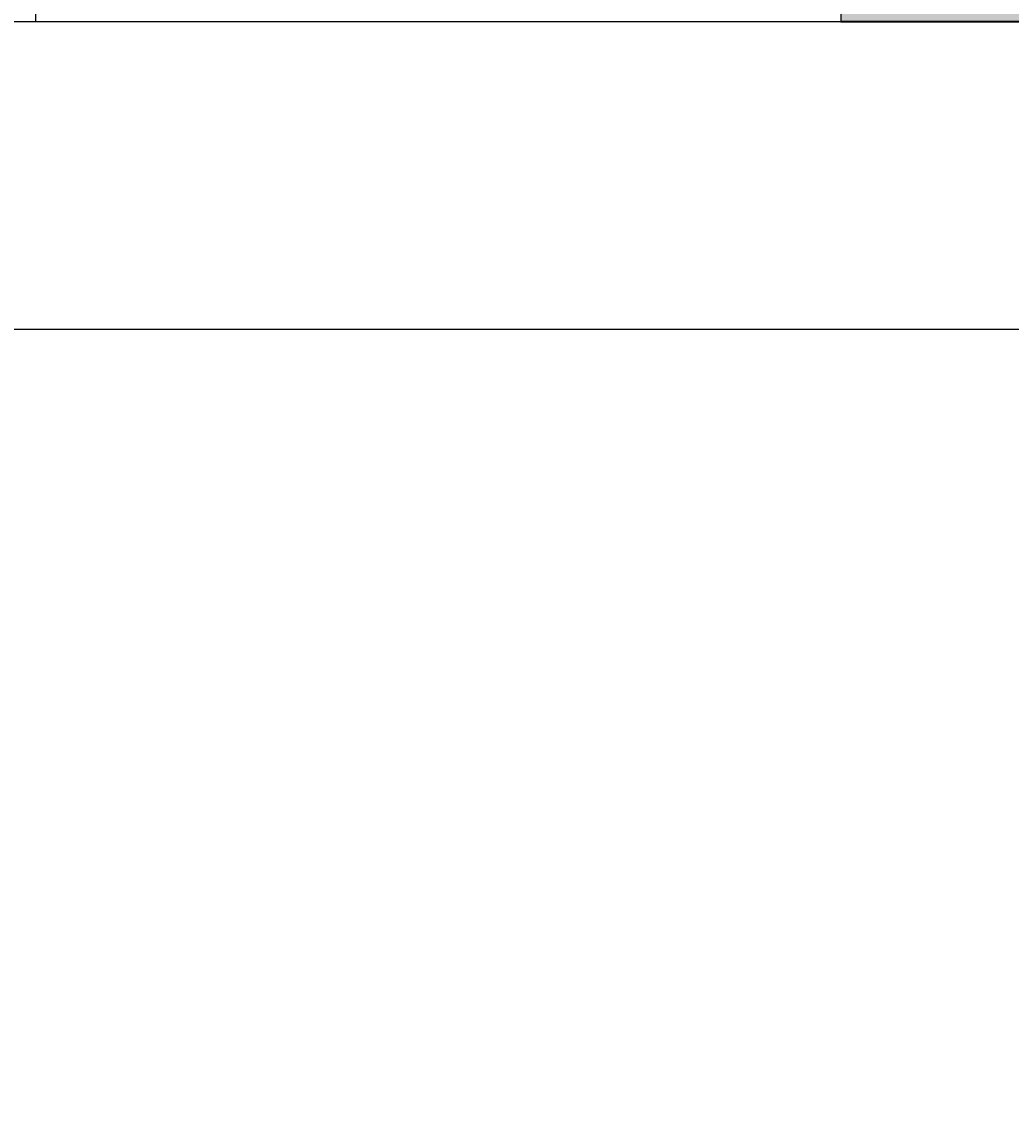
# Model space of a CAD drawing. Units: inches. Extents: x 1998 to 2588, y 1139 to 1977.
# Tile 98 of 134: x 2371 to 2397, y 1608 to 1637. Entities that reach past the tile are written whole.
import ezdxf

# ---------------------------------------------------------------- set-up
doc = ezdxf.new("R2010")
doc.units = ezdxf.units.IN
for name, color, linetype, lineweight in [('A-ANNO-DIMS', 2, 'Continuous', 18), ('A-WALL-PATT', 252, 'Continuous', 13), ('DOOR', 52, 'Continuous', 25), ('WALL', 200, 'Continuous', 35)]:
    doc.layers.add(name, color=color, linetype=linetype, lineweight=lineweight)
doc.styles.get("Standard").update_dxf_attribs({"font": 'arial.ttf'})
doc.dimstyles.get("Standard").update_dxf_attribs({"dimtxt": 0.18, "dimasz": 0.18, "dimexe": 0.18, "dimexo": 0.0625, "dimgap": 0.09, "dimtad": 0, "dimtih": 1, "dimtoh": 1, "dimdec": 4, "dimzin": 0, "dimdsep": 46, "dimtxsty": 'Standard', "dimcen": 0.09, "dimadec": 0, "dimazin": 0, "dimtfac": 1, "dimtdec": 4, "dimtofl": 0, "dimtmove": 0, "dimatfit": 3, "dimfxl": 1, "dimtolj": 1, "dimtzin": 0, "dimarcsym": 0})

# ---------------------------------------------------------------- blocks, each defined once
blk = doc.blocks.new('*U2')
for p, q in [((0, 0), (0, -6)), ((40, 0), (40, -6))]:
    blk.add_line(p, q)
blk.add_lwpolyline([(0, 0), (0, 40), (1.75, 40), (1.75, 0)], close=True)
blk.add_arc((0, 0), 40, 0, 90)
blk = doc.blocks.new('*D30')
at = {"layer": 'A-ANNO-DIMS', "color": 0, "lineweight": -2, "transparency": 16777216}
for p, q in [((2407.91, 1636.732), (1997.843, 1636.732)), ((1998.023, 1636.552), (1998.023, 1615.913)), ((1998.023, 1594.912), (1998.023, 1615.552)), ((2407.91, 1594.732), (1997.843, 1594.732))]:
    blk.add_line(p, q, dxfattribs=at)
at = {"layer": 'A-ANNO-DIMS', "color": 0, "transparency": 16777216}
for points in [[(1997.993, 1636.552), (1998.053, 1636.552), (1998.023, 1636.732)], [(1997.993, 1594.912), (1998.053, 1594.912), (1998.023, 1594.732)]]:
    blk.add_solid(points, dxfattribs=at)
at = {"layer": 'Defpoints', "color": 0, "transparency": 16777216}
for p in [(1998.023, 1636.732), (2407.973, 1636.732), (2407.973, 1594.732)]:
    blk.add_point(p, dxfattribs=at)
at = {"layer": 'A-ANNO-DIMS', "color": 0, "transparency": 16777216, "insert": (1998.023, 1615.732), "char_height": 0.18, "attachment_point": 5}
blk.add_mtext('\\A1;42', dxfattribs=at)
blk = doc.blocks.new('*D39')
at = {"layer": 'A-ANNO-DIMS', "color": 0, "lineweight": -2, "transparency": 16777216}
for p, q in [((2115.035, 1628.742), (2588.309, 1628.742)), ((2588.129, 1628.562), (2588.129, 1612.685)), ((2588.129, 1596.444), (2588.129, 1612.321)), ((2115.035, 1596.264), (2588.309, 1596.264))]:
    blk.add_line(p, q, dxfattribs=at)
at = {"layer": 'A-ANNO-DIMS', "color": 0, "transparency": 16777216}
for points in [[(2588.099, 1628.562), (2588.159, 1628.562), (2588.129, 1628.742)], [(2588.099, 1596.444), (2588.159, 1596.444), (2588.129, 1596.264)]]:
    blk.add_solid(points, dxfattribs=at)
at = {"layer": 'Defpoints', "color": 0, "transparency": 16777216}
for p in [(2114.973, 1628.742), (2588.129, 1628.742), (2114.973, 1596.264)]:
    blk.add_point(p, dxfattribs=at)
at = {"layer": 'A-ANNO-DIMS', "color": 0, "transparency": 16777216, "insert": (2588.129, 1612.503), "char_height": 0.18, "attachment_point": 5}
blk.add_mtext('\\A1;32.48', dxfattribs=at)

msp = doc.modelspace()

# ---------------------------------------------------------------- hatches: boundary and pattern name
at = {"layer": 'A-WALL-PATT'}
h = msp.add_hatch(color=256, dxfattribs=at)
h.dxf.hatch_style = 1
h.paths.add_polyline_path([(2527.4729, 1362.2324), (2510.9729, 1362.2324), (2510.9729, 1357.7324), (2518.4729, 1357.7324), (2518.4729, 1237.7324), (2503.1458, 1237.7324), (2503.1458, 1228.7324), (2527.4729, 1228.7324)])
h.paths.add_polyline_path([(2490.5682, 1362.2324), (2398.4729, 1362.2324), (2398.4729, 1357.7324), (2490.5682, 1357.7324)])
h.paths.add_polyline_path([(2224.9729, 1264.7324), (2222.9729, 1264.7324), (2222.9729, 1232.4125), (2341.4729, 1232.4125), (2341.4729, 1234.4125), (2224.9729, 1234.4125)])
h.paths.add_polyline_path([(2334.5332, 1273.7324), (2264.7638, 1273.7324), (2264.7638, 1269.5611, -0.043659), (2264.3413, 1264.7324), (2334.5332, 1264.7324)])
h.paths.add_polyline_path([(2236.9551, 1273.7324), (2234.4125, 1273.7324), (2234.4125, 1264.7324), (2236.9551, 1264.7324), (2236.9551, 1269.5611)])
h.paths.add_polyline_path([(2222.9729, 1293.2324), (2096.9729, 1293.2324), (2096.9729, 1345.0966), (2087.9729, 1345.0966), (2087.9729, 1284.2324), (2222.9729, 1284.2324), (2222.9729, 1285.137)])
h.paths.add_polyline_path([(2096.9729, 1458.7927), (2087.9729, 1458.7927), (2087.9729, 1417.7324), (2087.9729, 1413.2324), (2096.9729, 1413.2324), (2096.9729, 1417.7324)])
h.paths.add_polyline_path([(2096.9729, 1413.2324), (2087.9729, 1413.2324), (2087.9729, 1365.5012), (2096.9729, 1365.5012), (2096.9729, 1369.3358)])
h.paths.add_polyline_path([(2186.2943, 1417.7324), (2138.6074, 1417.7324), (2096.9729, 1417.7324), (2096.9729, 1413.2324), (2138.6074, 1413.2324), (2186.2943, 1413.2324)])
h.paths.add_polyline_path([(2181.4729, 1465.7324), (2176.9729, 1465.7324), (2176.9729, 1451.6434), (2181.4729, 1451.6434)])
h.paths.add_polyline_path([(2181.4729, 1422.1664), (2176.9729, 1422.1664), (2176.9729, 1417.7324), (2181.4729, 1417.7324)])
h.paths.add_polyline_path([(2063.9729, 1465.7324), (2087.9729, 1465.7324), (2087.9729, 1470.2324), (2059.4729, 1470.2324), (2059.4729, 1413.2324), (2087.9729, 1413.2324), (2087.9729, 1417.7324), (2063.9729, 1417.7324)])
h.paths.add_polyline_path([(2181.4729, 1755.2324), (2176.9729, 1755.2324), (2176.9729, 1748.6798), (2177.0513, 1748.6798), (2181.4729, 1748.6798)])
h.paths.add_polyline_path([(2227.4729, 1707.2324), (2220.4647, 1707.2324), (2220.4647, 1702.7324), (2222.9729, 1702.7324), (2222.9729, 1604.637), (2227.4729, 1604.637)])
h.paths.add_polyline_path([(2114.9729, 1702.7324), (2105.9729, 1702.7324), (2105.9729, 1628.4781, -0.0318759), (2110.1012, 1628.7416), (2114.9729, 1628.7416)])
h.paths.add_polyline_path([(2345.9729, 1739.3278), (2341.4729, 1739.3278), (2341.4729, 1647.5211), (2345.9729, 1647.5211)])
h.paths.add_polyline_path([(2350.6273, 1641.2324), (2345.9729, 1641.2324), (2345.9729, 1636.7324), (2350.6273, 1636.7324), (2350.6273, 1639.8729)])
h.paths.add_polyline_path([(2501.9729, 1641.2324), (2407.9729, 1641.2324), (2392.5005, 1641.2324), (2392.5005, 1639.8729), (2392.5005, 1636.7324), (2501.9729, 1636.7324)])
h.paths.add_polyline_path([(2510.9729, 1755.2324), (2501.9729, 1755.2324), (2501.9729, 1641.2324), (2510.9729, 1641.2324)])
h.paths.add_polyline_path([(2549.1786, 1641.2324), (2522.3775, 1641.2324), (2522.3775, 1636.7324), (2540.1786, 1636.7324), (2540.1786, 1480.7324), (2522.3775, 1480.7324), (2522.3775, 1476.2324), (2549.1786, 1476.2324)])
h.paths.add_polyline_path([(2498.1786, 1594.7324), (2407.9729, 1594.7324), (2407.9729, 1585.7324), (2416.9729, 1585.7324), (2489.1786, 1585.7324), (2489.1786, 1531.7324), (2416.9729, 1531.7324), (2407.9729, 1531.7324), (2407.9729, 1522.7324), (2498.1786, 1522.7324)])
h.paths.add_polyline_path([(2351.6437, 1480.7324), (2345.9729, 1480.7324), (2345.9729, 1476.2324), (2351.6437, 1476.2324), (2351.6437, 1477.5919)])
h.paths.add_polyline_path([(2501.9729, 1480.7324), (2498.1786, 1480.7324), (2407.9729, 1480.7324), (2393.5168, 1480.7324), (2393.5168, 1477.5919), (2393.5168, 1476.2324), (2501.9729, 1476.2324)])

# ---------------------------------------------------------------- linework, layer by layer
at = {"layer": 'WALL'}
msp.add_line((2501.9729, 1636.7324), (2392.5005, 1636.7324), dxfattribs=at)

# ---------------------------------------------------------------- block references
at = {"layer": 'DOOR', "yscale": 0.5234138920659225, "zscale": 0.5234138920659225}
for p, xscale in [((2350.6273, 1639.8729), 0.5234138920659225), ((2392.5005, 1639.8729), -0.5234138920659225)]:
    msp.add_blockref('*U2', p, dxfattribs=dict(at, xscale=xscale))

# ---------------------------------------------------------------- dimensions: what is measured, and where the dimension line sits
at = {"layer": 'A-ANNO-DIMS'}
for base, p1, p2, override, picture, middle in [((1998.0229, 1636.7324), (2407.9729, 1594.7324), (2407.9729, 1636.7324), {"dimdec": 0, "dimlfac": 1, "dimrnd": 0, "dimzin": 0, "dimdsep": 46, "dimlunit": 2}, '*D30', (1998.0229, 1615.7324)), ((2588.1286, 1628.7416), (2114.9729, 1596.2642), (2114.9729, 1628.7416), {"dimdec": 2, "dimlfac": 1, "dimrnd": 0, "dimzin": 0, "dimdsep": 46, "dimlunit": 2}, '*D39', (2588.1286, 1612.5029))]:
    dim = msp.add_linear_dim(base=base, p1=p1, p2=p2, angle=90, dimstyle='Standard', override=override, dxfattribs=at)
    dim.commit()
    dim.dimension.update_dxf_attribs({"geometry": picture, "text_midpoint": middle})

doc.saveas('drawing.dxf')
